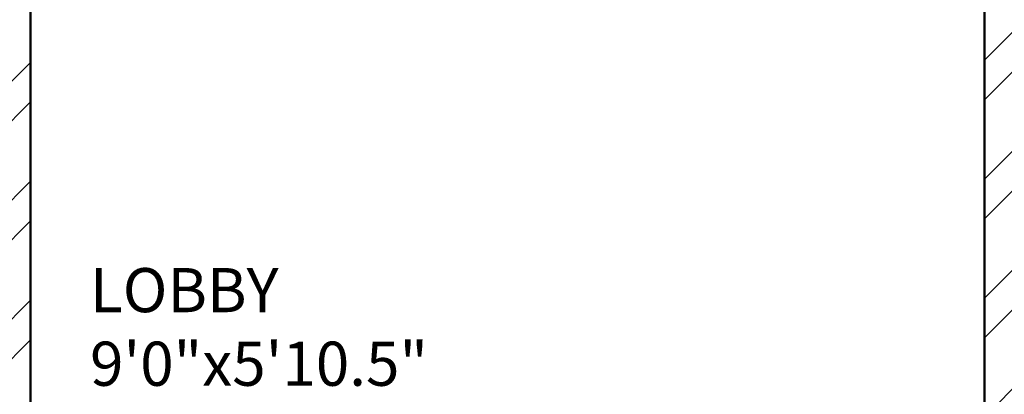
# Model space of a CAD drawing. Units: inches. Extents: x 963 to 2075, y 289 to 2657.
# Tile 68 of 98: x 1399 to 1511, y 2117 to 2160. Entities that reach past the tile are written whole.
import ezdxf

# ---------------------------------------------------------------- set-up
doc = ezdxf.new("R2010")
doc.units = ezdxf.units.IN
for name, color, linetype, lineweight in [('A-AREA-IDEN', 7, 'Continuous', 18), ('A-WALL', 7, 'Continuous', 50), ('A-WALL-PATT', 8, 'Continuous', 13)]:
    doc.layers.add(name, color=color, linetype=linetype, lineweight=lineweight)
doc.styles.get("Standard").update_dxf_attribs({"font": 'arial.ttf'})

msp = doc.modelspace()

# ---------------------------------------------------------------- hatches: boundary and pattern name
at = {"layer": 'A-WALL-PATT'}
h = msp.add_hatch(dxfattribs=at)
h.set_pattern_fill('ANSI32', color=256)
h.paths.add_polyline_path([(1296.92, 2558.32), (1203.92, 2558.32), (1203.92, 2493.82), (1191.53, 2493.82), (1191.53, 2489.32), (1211.06, 2489.32), (1211.06, 2492.02), (1211.06, 2493.82), (1208.42, 2493.82), (1208.42, 2553.82), (1292.42, 2553.82), (1292.42, 2538.86), (1296.92, 2538.86)])
h.paths.add_polyline_path([(1442.42, 2558.32), (1349.42, 2558.32), (1349.42, 2538.94), (1353.92, 2538.94), (1353.92, 2553.82), (1437.92, 2553.82), (1437.92, 2493.82), (1434.54, 2493.82), (1434.54, 2489.32), (1448.31, 2489.32), (1448.31, 2491.57), (1448.31, 2493.82), (1442.42, 2493.82)])
h.paths.add_polyline_path([(1415.55, 2491.57), (1415.55, 2493.82), (1340.94, 2493.82), (1340.94, 2489.32), (1371.92, 2489.32), (1371.92, 2378.32), (1367.6, 2378.32), (1367.6, 2373.82), (1371.92, 2373.82), (1371.92, 2355.19), (1376.42, 2355.19), (1376.42, 2489.32), (1415.55, 2489.32)])
h.paths.add_polyline_path([(1304.94, 2491.57), (1304.94, 2493.82), (1296.92, 2493.82), (1296.92, 2514.86), (1292.42, 2514.86), (1292.42, 2493.82), (1232.81, 2493.82), (1232.81, 2489.32), (1256.42, 2489.32), (1256.42, 2327.32), (1253.71, 2327.32), (1253.71, 2322.82), (1328.42, 2322.82), (1328.42, 2331.15), (1323.92, 2331.15), (1323.92, 2327.32), (1260.92, 2327.32), (1260.92, 2373.82), (1323.92, 2373.82), (1323.92, 2357.81), (1328.42, 2357.81), (1328.42, 2373.82), (1346.01, 2373.82), (1346.01, 2376.07), (1346.01, 2378.32), (1260.92, 2378.32), (1260.92, 2489.32), (1304.94, 2489.32)])
h.paths.add_polyline_path([(1226.65, 2327.32), (1124.42, 2327.32), (1124.42, 2347.45), (1119.92, 2347.45), (1119.92, 2322.82), (1163.42, 2322.82), (1163.42, 2305.43), (1165.67, 2305.43), (1167.92, 2305.43), (1167.92, 2322.82), (1226.65, 2322.82), (1226.65, 2325.07)])
h.paths.add_polyline_path([(1095.92, 2489.32), (1124.42, 2489.32), (1131.53, 2489.32), (1131.53, 2491.57), (1131.53, 2493.82), (1119.92, 2493.82), (1091.42, 2493.82), (1091.42, 2417.32), (1095.92, 2417.32), (1119.92, 2417.32), (1119.92, 2407.45), (1124.42, 2407.45), (1124.42, 2421.82), (1095.92, 2421.82)])
h.paths.add_polyline_path([(1512.92, 2558.32), (1508.42, 2558.32), (1508.42, 2493.82), (1503.4, 2493.82), (1503.4, 2489.32), (1508.42, 2489.32), (1508.42, 2327.32), (1376.42, 2327.32), (1376.42, 2330.27), (1371.92, 2330.27), (1371.92, 2298.74), (1376.42, 2298.74), (1376.42, 2322.82), (1508.42, 2322.82), (1508.42, 2165.32), (1504.26, 2165.32), (1504.26, 2160.82), (1508.42, 2160.82), (1508.42, 2108.32), (1512.92, 2108.32), (1512.92, 2160.82), (1516.18, 2160.82), (1516.18, 2163.07), (1516.18, 2165.32), (1512.92, 2165.32), (1512.92, 2322.82), (1644.92, 2322.82), (1644.92, 2298.74), (1649.42, 2298.74), (1649.42, 2322.82), (1649.42, 2330.94), (1647.17, 2330.94), (1644.92, 2330.94), (1644.92, 2327.32), (1512.92, 2327.32), (1512.92, 2489.32), (1516.76, 2489.32), (1516.76, 2491.57), (1516.76, 2493.82), (1512.92, 2493.82)])
h.paths.add_polyline_path([(1671.92, 2558.32), (1578.92, 2558.32), (1578.92, 2493.82), (1573.53, 2493.82), (1573.53, 2489.32), (1586.54, 2489.32), (1586.54, 2491.57), (1586.54, 2493.82), (1583.42, 2493.82), (1583.42, 2553.82), (1667.42, 2553.82), (1667.42, 2541.11), (1671.92, 2541.11)])
h.paths.add_polyline_path([(1681.26, 2493.82), (1671.92, 2493.82), (1671.92, 2517.11), (1667.42, 2517.11), (1667.42, 2493.82), (1610.22, 2493.82), (1610.22, 2489.32), (1644.92, 2489.32), (1644.92, 2357.87), (1649.42, 2357.87), (1649.42, 2373.82), (1652.2, 2373.82), (1652.2, 2375.83), (1652.2, 2378.32), (1649.42, 2378.32), (1649.42, 2489.32), (1681.26, 2489.32), (1681.26, 2491.57)])
h.paths.add_polyline_path([(1821.92, 2558.32), (1728.92, 2558.32), (1728.92, 2541), (1733.42, 2541), (1733.42, 2553.82), (1817.42, 2553.82), (1817.42, 2493.82), (1813.51, 2493.82), (1813.51, 2489.32), (1830.08, 2489.32), (1830.08, 2491.57), (1830.08, 2493.82), (1821.92, 2493.82)])
h.paths.add_polyline_path([(1794.24, 2493.82), (1717.26, 2493.82), (1717.26, 2489.32), (1760.42, 2489.32), (1760.42, 2378.32), (1674.4, 2378.32), (1674.4, 2373.82), (1692.92, 2373.82), (1692.92, 2356.95), (1697.42, 2356.95), (1697.42, 2373.82), (1760.42, 2373.82), (1760.42, 2327.32), (1697.42, 2327.32), (1697.42, 2333.34), (1692.92, 2333.34), (1692.92, 2322.82), (1768.04, 2322.82), (1768.04, 2325.07), (1768.04, 2327.32), (1764.92, 2327.32), (1764.92, 2489.32), (1794.24, 2489.32)])
h.paths.add_polyline_path([(1733.42, 2517), (1728.92, 2517), (1728.92, 2493.82), (1733.42, 2493.82)], flags=17)
h.paths.add_polyline_path([(1929.92, 2493.82), (1890.08, 2493.82), (1890.08, 2489.32), (1896.92, 2489.32), (1925.42, 2489.32), (1925.42, 2421.82), (1896.92, 2421.82), (1896.92, 2408.32), (1901.42, 2408.32), (1901.42, 2417.32), (1925.42, 2417.32), (1929.92, 2417.32)])
h.paths.add_polyline_path([(1901.42, 2348.32), (1896.92, 2348.32), (1896.92, 2327.32), (1800.42, 2327.32), (1800.42, 2322.82), (1853.42, 2322.82), (1853.42, 2309.45), (1857.92, 2309.45), (1857.92, 2322.82), (1901.42, 2322.82)])
h.paths.add_polyline_path([(1857.92, 2249.45), (1853.42, 2249.45), (1853.42, 2214.82), (1686.31, 2214.82), (1686.31, 2210.32), (1853.42, 2210.32), (1853.42, 2202.13), (1857.92, 2202.13), (1857.92, 2210.32)])
h.paths.add_polyline_path([(1857.92, 2142.13), (1853.42, 2142.13), (1853.42, 2115.42), (1841.42, 2115.42), (1841.42, 2088.53), (1841.42, 2046.95), (1845.92, 2046.95), (1845.92, 2110.92), (1905.92, 2110.92), (1905.92, 2092.52), (1910.42, 2092.52), (1910.42, 2115.42), (1857.92, 2115.42)])
h.paths.add_polyline_path([(1532.44, 1482.34), (1573.46, 1482.34), (1573.46, 1501), (1532.44, 1501)], flags=9)
h.paths.add_polyline_path([(1438.66, 1486.3), (1479.68, 1486.3), (1479.68, 1504.96), (1438.66, 1504.96)], flags=9)
h.paths.add_polyline_path([(1411.22, 1365.31), (1659.14, 1365.31), (1659.14, 1402.4), (1411.22, 1402.4)], flags=9)
h.paths.add_polyline_path([(1185.67, 2296.3), (1248.16, 2296.3), (1248.16, 2314.95), (1185.67, 2314.95)], flags=9)
h.paths.add_polyline_path([(1177.31, 2187.35), (1216.15, 2187.35), (1216.15, 2206.01), (1177.31, 2206.01)], flags=9)
h.paths.add_polyline_path([(1295.1, 1602.08), (1328.26, 1602.08), (1328.26, 1620.74), (1295.1, 1620.74)], flags=9)
h.paths.add_polyline_path([(1525.13, 2005.99), (1558.39, 2005.99), (1558.39, 2024.65), (1525.13, 2024.65)], flags=9)
h.paths.add_polyline_path([(1459.61, 1977.13), (1472.19, 1977.13), (1472.19, 1987.43), (1459.61, 1987.43)], flags=9)
h.paths.add_polyline_path([(1467.81, 2053.68), (1480.02, 2053.68), (1480.02, 2063.98), (1467.81, 2063.98)], flags=9)
h.paths.add_polyline_path([(1555.18, 2119.02), (1584.56, 2119.02), (1584.56, 2137.68), (1555.18, 2137.68)], flags=25)
h.paths.add_polyline_path([(1405.39, 2115.29), (1444.48, 2115.29), (1444.48, 2133.95), (1405.39, 2133.95)], flags=25)
h.paths.add_polyline_path([(1698.48, 2004.26), (1727.69, 2004.26), (1727.69, 2022.92), (1698.48, 2022.92)], flags=9)
h.paths.add_polyline_path([(1612.16, 1972.86), (1629.02, 1972.86), (1629.02, 1983.16), (1612.16, 1983.16)], flags=9)
h.paths.add_polyline_path([(1608.29, 2060.04), (1625.15, 2060.04), (1625.15, 2070.34), (1608.29, 2070.34)], flags=9)
h.paths.add_polyline_path([(1527.95, 1684.4), (1566.79, 1684.4), (1566.79, 1703.06), (1527.95, 1703.06)], flags=9)
h.paths.add_polyline_path([(1422.79, 1683.59), (1461.63, 1683.59), (1461.63, 1702.25), (1422.79, 1702.25)], flags=9)
h.paths.add_polyline_path([(1531.26, 1732.46), (1574.01, 1732.46), (1574.01, 1751.12), (1531.26, 1751.12)], flags=9)
h.paths.add_polyline_path([(1402.87, 1732.85), (1439.8, 1732.85), (1439.8, 1751.5), (1402.87, 1751.5)], flags=9)
h.paths.add_polyline_path([(1243.12, 1923.13), (1281.96, 1923.13), (1281.96, 1941.79), (1243.12, 1941.79)], flags=9)
h.paths.add_polyline_path([(1181.75, 1792.27), (1244.24, 1792.27), (1244.24, 1810.93), (1181.75, 1810.93)], flags=9)
h.paths.add_polyline_path([(1265.82, 1670.3), (1316.07, 1670.3), (1316.07, 1688.96), (1265.82, 1688.96)], flags=9)
h.paths.add_polyline_path([(1140.26, 1676.05), (1179.1, 1676.05), (1179.1, 1694.71), (1140.26, 1694.71)], flags=9)
h.paths.add_polyline_path([(1107.49, 1490.89), (1143.37, 1490.89), (1143.37, 1509.55), (1107.49, 1509.55)], flags=9)
h.paths.add_polyline_path([(1217.58, 1483.9), (1246.74, 1483.9), (1246.74, 1502.56), (1217.58, 1502.56)], flags=9)
h.paths.add_polyline_path([(1389.21, 1486.92), (1418.37, 1486.92), (1418.37, 1505.58), (1389.21, 1505.58)], flags=9)
h.paths.add_polyline_path([(1672.21, 1602.08), (1705.37, 1602.08), (1705.37, 1620.74), (1672.21, 1620.74)], flags=9)
h.paths.add_polyline_path([(1752.08, 1522.64), (1781.24, 1522.64), (1781.24, 1541.3), (1752.08, 1541.3)], flags=9)
h.paths.add_polyline_path([(1848.27, 1491.26), (1884.16, 1491.26), (1884.16, 1509.92), (1848.27, 1509.92)], flags=9)
h.paths.add_polyline_path([(1822.47, 1685.62), (1861.31, 1685.62), (1861.31, 1704.28), (1822.47, 1704.28)], flags=9)
h.paths.add_polyline_path([(1713.19, 1672.23), (1763.44, 1672.23), (1763.44, 1690.89), (1713.19, 1690.89)], flags=9)
h.paths.add_polyline_path([(1736.62, 1790.58), (1799.11, 1790.58), (1799.11, 1809.24), (1736.62, 1809.24)], flags=9)
h.paths.add_polyline_path([(1691.49, 1916.36), (1730.33, 1916.36), (1730.33, 1935.01), (1691.49, 1935.01)], flags=9)
h.paths.add_polyline_path([(1764.87, 1973.92), (1794.31, 1973.92), (1794.31, 1992.58), (1764.87, 1992.58)], flags=9)
h.paths.add_polyline_path([(1767.85, 2034.02), (1797.29, 2034.02), (1797.29, 2052.67), (1767.85, 2052.67)], flags=9)
h.paths.add_polyline_path([(1851.59, 2060.33), (1880.75, 2060.33), (1880.75, 2078.99), (1851.59, 2078.99)], flags=25)
h.paths.add_polyline_path([(1688.49, 2086.87), (1727.33, 2086.87), (1727.33, 2105.53), (1688.49, 2105.53)], flags=9)
h.paths.add_polyline_path([(1537.74, 2293.58), (1580.49, 2293.58), (1580.49, 2312.24), (1537.74, 2312.24)], flags=25)
h.paths.add_polyline_path([(1425.59, 2296.11), (1468.34, 2296.11), (1468.34, 2314.77), (1425.59, 2314.77)], flags=25)
h.paths.add_polyline_path([(1278.52, 2004.18), (1307.72, 2004.18), (1307.72, 2022.84), (1278.52, 2022.84)], flags=9)
h.paths.add_polyline_path([(1193.28, 1973.63), (1222.72, 1973.63), (1222.72, 1992.29), (1193.28, 1992.29)], flags=9)
h.paths.add_polyline_path([(1192.41, 2040.58), (1221.84, 2040.58), (1221.84, 2059.23), (1192.41, 2059.23)], flags=9)
h.paths.add_polyline_path([(1130.6, 1951.39), (1159.76, 1951.39), (1159.76, 1970.05), (1130.6, 1970.05)], flags=9)
h.paths.add_polyline_path([(1132.83, 2052.49), (1161.98, 2052.49), (1161.98, 2071.15), (1132.83, 2071.15)], flags=9)
h.paths.add_polyline_path([(1265.13, 2334.62), (1315.38, 2334.62), (1315.38, 2353.28), (1265.13, 2353.28)], flags=25)
h.paths.add_polyline_path([(1136.74, 2330.79), (1175.58, 2330.79), (1175.58, 2349.44), (1136.74, 2349.44)], flags=9)
h.paths.add_polyline_path([(1287.42, 2417.2), (1320.58, 2417.2), (1320.58, 2435.86), (1287.42, 2435.86)], flags=25)
h.paths.add_polyline_path([(1430.99, 2329.16), (1469.83, 2329.16), (1469.83, 2347.82), (1430.99, 2347.82)], flags=25)
h.paths.add_polyline_path([(1525.42, 2329.21), (1564.26, 2329.21), (1564.26, 2347.87), (1525.42, 2347.87)], flags=25)
h.paths.add_polyline_path([(1684.52, 2382.8), (1717.68, 2382.8), (1717.68, 2401.46), (1684.52, 2401.46)], flags=25)
h.paths.add_polyline_path([(1704.81, 2340.29), (1755.05, 2340.29), (1755.05, 2358.95), (1704.81, 2358.95)], flags=25)
h.paths.add_polyline_path([(1694.11, 2287.76), (1756.6, 2287.76), (1756.6, 2306.41), (1694.11, 2306.41)], flags=9)
h.paths.add_polyline_path([(1815.78, 2329.86), (1854.62, 2329.86), (1854.62, 2348.52), (1815.78, 2348.52)], flags=9)
h.paths.add_polyline_path([(1842.87, 2514.26), (1878.76, 2514.26), (1878.76, 2532.91), (1842.87, 2532.91)], flags=9)
h.paths.add_polyline_path([(1769.51, 2531.45), (1798.67, 2531.45), (1798.67, 2550.1), (1769.51, 2550.1)], flags=25)
h.paths.add_polyline_path([(1594.77, 2518.47), (1623.93, 2518.47), (1623.93, 2537.13), (1594.77, 2537.13)], flags=25)
h.paths.add_polyline_path([(1520.72, 2516.18), (1556.61, 2516.18), (1556.61, 2534.84), (1520.72, 2534.84)], flags=25)
h.paths.add_polyline_path([(1464.46, 2516.69), (1500.34, 2516.69), (1500.34, 2535.35), (1464.46, 2535.35)], flags=25)
h.paths.add_polyline_path([(1365.7, 2528.97), (1394.85, 2528.97), (1394.85, 2547.63), (1365.7, 2547.63)], flags=25)
h.paths.add_polyline_path([(1222.84, 2516.23), (1252, 2516.23), (1252, 2534.89), (1222.84, 2534.89)], flags=25)
h.paths.add_polyline_path([(1104.55, 2509.6), (1140.43, 2509.6), (1140.43, 2528.26), (1104.55, 2528.26)], flags=9)
h = msp.add_hatch(dxfattribs=at)
h.set_pattern_fill('ANSI32', color=256)
h.paths.add_polyline_path([(1335.97, 2212.57), (1335.97, 2214.82), (1167.92, 2214.82), (1167.92, 2245.43), (1163.42, 2245.43), (1163.42, 2210.32), (1163.42, 2194.81), (1167.92, 2194.81), (1167.92, 2210.32), (1335.97, 2210.32)])
h.paths.add_polyline_path([(1532.44, 1482.34), (1573.46, 1482.34), (1573.46, 1501), (1532.44, 1501)], flags=9)
h.paths.add_polyline_path([(1438.66, 1486.3), (1479.68, 1486.3), (1479.68, 1504.96), (1438.66, 1504.96)], flags=9)
h.paths.add_polyline_path([(1411.22, 1365.31), (1659.14, 1365.31), (1659.14, 1402.4), (1411.22, 1402.4)], flags=9)
h.paths.add_polyline_path([(1185.67, 2296.3), (1248.16, 2296.3), (1248.16, 2314.95), (1185.67, 2314.95)], flags=9)
h.paths.add_polyline_path([(1177.31, 2187.35), (1216.15, 2187.35), (1216.15, 2206.01), (1177.31, 2206.01)], flags=9)
h.paths.add_polyline_path([(1295.1, 1602.08), (1328.26, 1602.08), (1328.26, 1620.74), (1295.1, 1620.74)], flags=9)
h.paths.add_polyline_path([(1525.13, 2005.99), (1558.39, 2005.99), (1558.39, 2024.65), (1525.13, 2024.65)], flags=9)
h.paths.add_polyline_path([(1459.61, 1977.13), (1472.19, 1977.13), (1472.19, 1987.43), (1459.61, 1987.43)], flags=9)
h.paths.add_polyline_path([(1467.81, 2053.68), (1480.02, 2053.68), (1480.02, 2063.98), (1467.81, 2063.98)], flags=9)
h.paths.add_polyline_path([(1555.18, 2119.02), (1584.56, 2119.02), (1584.56, 2137.68), (1555.18, 2137.68)], flags=9)
h.paths.add_polyline_path([(1405.39, 2115.29), (1444.48, 2115.29), (1444.48, 2133.95), (1405.39, 2133.95)], flags=9)
h.paths.add_polyline_path([(1698.48, 2004.26), (1727.69, 2004.26), (1727.69, 2022.92), (1698.48, 2022.92)], flags=9)
h.paths.add_polyline_path([(1612.16, 1972.86), (1629.02, 1972.86), (1629.02, 1983.16), (1612.16, 1983.16)], flags=9)
h.paths.add_polyline_path([(1608.29, 2060.04), (1625.15, 2060.04), (1625.15, 2070.34), (1608.29, 2070.34)], flags=9)
h.paths.add_polyline_path([(1527.95, 1684.4), (1566.79, 1684.4), (1566.79, 1703.06), (1527.95, 1703.06)], flags=9)
h.paths.add_polyline_path([(1422.79, 1683.59), (1461.63, 1683.59), (1461.63, 1702.25), (1422.79, 1702.25)], flags=9)
h.paths.add_polyline_path([(1531.26, 1732.46), (1574.01, 1732.46), (1574.01, 1751.12), (1531.26, 1751.12)], flags=9)
h.paths.add_polyline_path([(1402.87, 1732.85), (1439.8, 1732.85), (1439.8, 1751.5), (1402.87, 1751.5)], flags=9)
h.paths.add_polyline_path([(1243.12, 1923.13), (1281.96, 1923.13), (1281.96, 1941.79), (1243.12, 1941.79)], flags=9)
h.paths.add_polyline_path([(1181.75, 1792.27), (1244.24, 1792.27), (1244.24, 1810.93), (1181.75, 1810.93)], flags=9)
h.paths.add_polyline_path([(1265.82, 1670.3), (1316.07, 1670.3), (1316.07, 1688.96), (1265.82, 1688.96)], flags=9)
h.paths.add_polyline_path([(1140.26, 1676.05), (1179.1, 1676.05), (1179.1, 1694.71), (1140.26, 1694.71)], flags=9)
h.paths.add_polyline_path([(1107.49, 1490.89), (1143.37, 1490.89), (1143.37, 1509.55), (1107.49, 1509.55)], flags=9)
h.paths.add_polyline_path([(1217.58, 1483.9), (1246.74, 1483.9), (1246.74, 1502.56), (1217.58, 1502.56)], flags=9)
h.paths.add_polyline_path([(1389.21, 1486.92), (1418.37, 1486.92), (1418.37, 1505.58), (1389.21, 1505.58)], flags=9)
h.paths.add_polyline_path([(1672.21, 1602.08), (1705.37, 1602.08), (1705.37, 1620.74), (1672.21, 1620.74)], flags=9)
h.paths.add_polyline_path([(1752.08, 1522.64), (1781.24, 1522.64), (1781.24, 1541.3), (1752.08, 1541.3)], flags=9)
h.paths.add_polyline_path([(1848.27, 1491.26), (1884.16, 1491.26), (1884.16, 1509.92), (1848.27, 1509.92)], flags=9)
h.paths.add_polyline_path([(1822.47, 1685.62), (1861.31, 1685.62), (1861.31, 1704.28), (1822.47, 1704.28)], flags=9)
h.paths.add_polyline_path([(1713.19, 1672.23), (1763.44, 1672.23), (1763.44, 1690.89), (1713.19, 1690.89)], flags=9)
h.paths.add_polyline_path([(1736.62, 1790.58), (1799.11, 1790.58), (1799.11, 1809.24), (1736.62, 1809.24)], flags=9)
h.paths.add_polyline_path([(1691.49, 1916.36), (1730.33, 1916.36), (1730.33, 1935.01), (1691.49, 1935.01)], flags=9)
h.paths.add_polyline_path([(1764.87, 1973.92), (1794.31, 1973.92), (1794.31, 1992.58), (1764.87, 1992.58)], flags=9)
h.paths.add_polyline_path([(1767.85, 2034.02), (1797.29, 2034.02), (1797.29, 2052.67), (1767.85, 2052.67)], flags=9)
h.paths.add_polyline_path([(1851.59, 2060.33), (1880.75, 2060.33), (1880.75, 2078.99), (1851.59, 2078.99)], flags=9)
h.paths.add_polyline_path([(1688.49, 2086.87), (1727.33, 2086.87), (1727.33, 2105.53), (1688.49, 2105.53)], flags=9)
h.paths.add_polyline_path([(1537.74, 2293.58), (1580.49, 2293.58), (1580.49, 2312.24), (1537.74, 2312.24)], flags=9)
h.paths.add_polyline_path([(1425.59, 2296.11), (1468.34, 2296.11), (1468.34, 2314.77), (1425.59, 2314.77)], flags=9)
h.paths.add_polyline_path([(1278.52, 2004.18), (1307.72, 2004.18), (1307.72, 2022.84), (1278.52, 2022.84)], flags=9)
h.paths.add_polyline_path([(1193.28, 1973.63), (1222.72, 1973.63), (1222.72, 1992.29), (1193.28, 1992.29)], flags=9)
h.paths.add_polyline_path([(1192.41, 2040.58), (1221.84, 2040.58), (1221.84, 2059.23), (1192.41, 2059.23)], flags=9)
h.paths.add_polyline_path([(1130.6, 1951.39), (1159.76, 1951.39), (1159.76, 1970.05), (1130.6, 1970.05)], flags=9)
h.paths.add_polyline_path([(1132.83, 2052.49), (1161.98, 2052.49), (1161.98, 2071.15), (1132.83, 2071.15)], flags=9)
h.paths.add_polyline_path([(1265.13, 2334.62), (1315.38, 2334.62), (1315.38, 2353.28), (1265.13, 2353.28)], flags=9)
h.paths.add_polyline_path([(1136.74, 2330.79), (1175.58, 2330.79), (1175.58, 2349.44), (1136.74, 2349.44)], flags=9)
h.paths.add_polyline_path([(1287.42, 2417.2), (1320.58, 2417.2), (1320.58, 2435.86), (1287.42, 2435.86)], flags=9)
h.paths.add_polyline_path([(1430.99, 2329.16), (1469.83, 2329.16), (1469.83, 2347.82), (1430.99, 2347.82)], flags=9)
h.paths.add_polyline_path([(1525.42, 2329.21), (1564.26, 2329.21), (1564.26, 2347.87), (1525.42, 2347.87)], flags=9)
h.paths.add_polyline_path([(1684.52, 2382.8), (1717.68, 2382.8), (1717.68, 2401.46), (1684.52, 2401.46)], flags=9)
h.paths.add_polyline_path([(1704.81, 2340.29), (1755.05, 2340.29), (1755.05, 2358.95), (1704.81, 2358.95)], flags=9)
h.paths.add_polyline_path([(1694.11, 2287.76), (1756.6, 2287.76), (1756.6, 2306.41), (1694.11, 2306.41)], flags=9)
h.paths.add_polyline_path([(1815.78, 2329.86), (1854.62, 2329.86), (1854.62, 2348.52), (1815.78, 2348.52)], flags=9)
h.paths.add_polyline_path([(1842.87, 2514.26), (1878.76, 2514.26), (1878.76, 2532.91), (1842.87, 2532.91)], flags=9)
h.paths.add_polyline_path([(1769.51, 2531.45), (1798.67, 2531.45), (1798.67, 2550.1), (1769.51, 2550.1)], flags=9)
h.paths.add_polyline_path([(1594.77, 2518.47), (1623.93, 2518.47), (1623.93, 2537.13), (1594.77, 2537.13)], flags=9)
h.paths.add_polyline_path([(1520.72, 2516.18), (1556.61, 2516.18), (1556.61, 2534.84), (1520.72, 2534.84)], flags=9)
h.paths.add_polyline_path([(1464.46, 2516.69), (1500.34, 2516.69), (1500.34, 2535.35), (1464.46, 2535.35)], flags=9)
h.paths.add_polyline_path([(1365.7, 2528.97), (1394.85, 2528.97), (1394.85, 2547.63), (1365.7, 2547.63)], flags=9)
h.paths.add_polyline_path([(1222.84, 2516.23), (1252, 2516.23), (1252, 2534.89), (1222.84, 2534.89)], flags=9)
h.paths.add_polyline_path([(1104.55, 2509.6), (1140.43, 2509.6), (1140.43, 2528.26), (1104.55, 2528.26)], flags=9)
h = msp.add_hatch(dxfattribs=at)
h.set_pattern_fill('ANSI32', color=256)
h.paths.add_polyline_path([(1473.61, 2163.07), (1473.61, 2165.32), (1376.42, 2165.32), (1376.42, 2227.98), (1371.92, 2227.98), (1371.92, 2214.82), (1368.41, 2214.82), (1368.41, 2210.32), (1371.92, 2210.32), (1371.92, 2160.82), (1395.92, 2160.82), (1395.92, 2090.32), (1217.34, 2090.32), (1217.34, 2085.82), (1395.92, 2085.82), (1458.92, 2085.82), (1458.92, 2108.32), (1454.42, 2108.32), (1454.42, 2090.32), (1400.42, 2090.32), (1400.42, 2160.82), (1473.61, 2160.82)])
h.paths.add_polyline_path([(1649.42, 2210.32), (1653.23, 2210.32), (1653.23, 2214.82), (1649.42, 2214.82), (1649.42, 2227.98), (1644.92, 2227.98), (1644.92, 2165.32), (1550.1, 2165.32), (1550.1, 2160.82), (1620.92, 2160.82), (1620.92, 2112.82), (1555.45, 2112.82), (1555.45, 2108.32), (1584.33, 2108.32), (1584.33, 2084.92), (1588.83, 2084.92), (1588.83, 2108.32), (1625.42, 2108.32), (1667.95, 2108.32), (1667.95, 2022.67), (1588.83, 2022.67), (1588.83, 2047.41), (1584.33, 2047.41), (1584.33, 1996), (1588.83, 1996), (1588.83, 2018.32), (1667.95, 2018.17), (1667.95, 1928.32), (1625.42, 1928.32), (1625.42, 1923.82), (1672.45, 1923.82), (1672.45, 1928.32), (1672.45, 1946.66), (1785.45, 1946.66), (1785.45, 1951.16), (1743.03, 1951.16), (1743.03, 2017.92), (1841.42, 2017.92), (1841.42, 2014.77), (1845.92, 2014.77), (1845.92, 2017.92), (1905.92, 2017.92), (1905.92, 1987.51), (1910.42, 1987.51), (1910.42, 2022.42), (1910.42, 2068.52), (1905.92, 2068.52), (1905.92, 2022.42), (1845.92, 2022.42), (1845.92, 2025.85), (1843.67, 2025.85), (1841.42, 2025.85), (1841.42, 2022.42), (1743.03, 2022.42), (1743.03, 2084.03), (1768.45, 2084.03), (1785.45, 2084.03), (1785.45, 2088.53), (1672.45, 2088.53), (1672.45, 2112.82), (1667.95, 2112.82), (1625.42, 2112.82), (1625.42, 2160.82), (1649.42, 2160.82)])
h.paths.add_polyline_path([(1672.45, 2084.03), (1738.53, 2084.03), (1738.53, 1951.16), (1672.45, 1951.16)], flags=16)
h.paths.add_polyline_path([(1672.45, 2084.03), (1738.53, 2084.03), (1705.49, 2017.6)], flags=0)
h.paths.add_polyline_path([(1262.77, 2085.82), (1258.27, 2085.82), (1258.27, 2023.28), (1184.42, 2023.28), (1184.42, 2018.78), (1258.27, 2018.78), (1258.27, 1950.82), (1262.77, 1950.82)])
h.paths.add_polyline_path([(1312.27, 2085.82), (1307.77, 2085.82), (1307.77, 1950.82), (1312.27, 1950.82)])
h.paths.add_polyline_path([(1458.92, 1950.82), (1395.92, 1950.82), (1216.57, 1950.82), (1216.57, 1946.32), (1346.42, 1946.32), (1395.92, 1946.32), (1395.92, 1875.82), (1371.92, 1875.82), (1371.92, 1826.32), (1368.93, 1826.32), (1368.93, 1821.82), (1371.92, 1821.82), (1371.92, 1813.62), (1376.42, 1813.62), (1376.42, 1871.32), (1474.5, 1871.32), (1474.5, 1873.57), (1474.5, 1875.82), (1400.42, 1875.82), (1400.42, 1946.32), (1454.42, 1946.32), (1454.42, 1928.32), (1458.92, 1928.32)])
h.paths.add_polyline_path([(1184.42, 2120.78), (1167.92, 2120.78), (1167.92, 2134.81), (1165.67, 2134.81), (1163.42, 2134.81), (1163.42, 2120.78), (1119.92, 2120.78), (1119.92, 2098.1), (1124.42, 2098.1), (1124.42, 2116.28), (1167.92, 2116.28), (1179.92, 2116.28), (1179.92, 2045.92), (1184.42, 2045.92), (1184.42, 2090.32), (1184.42, 2116.28)])
h.paths.add_polyline_path([(1124.42, 2018.78), (1179.92, 2018.78), (1179.92, 2016.29), (1184.42, 2016.29), (1184.42, 2023.28), (1184.42, 2026.59), (1182.17, 2026.59), (1179.92, 2026.59), (1179.92, 2023.28), (1124.42, 2023.28), (1124.42, 2074.1), (1119.92, 2074.1), (1119.92, 2018.78), (1119.92, 1979.63), (1124.42, 1979.63)])
h.paths.add_polyline_path([(1184.42, 1925.78), (1184.42, 1946.32), (1184.42, 1996.07), (1182.17, 1996.07), (1179.92, 1996.07), (1179.92, 1925.78), (1124.42, 1925.78), (1124.42, 1955.63), (1119.92, 1955.5), (1119.92, 1921.28), (1158.92, 1921.28), (1158.92, 1909.98), (1163.42, 1909.98), (1163.42, 1921.28), (1184.42, 1921.28)])
h.paths.add_polyline_path([(1341.45, 1826.32), (1163.42, 1826.32), (1163.42, 1849.98), (1158.92, 1849.98), (1158.92, 1821.82), (1158.92, 1804.03), (1163.42, 1804.03), (1163.42, 1821.82), (1341.45, 1821.82)])
h.paths.add_polyline_path([(1222.98, 1713.82), (1163.42, 1713.82), (1163.42, 1744.03), (1161.17, 1744.03), (1158.92, 1744.03), (1158.92, 1713.82), (1119.92, 1713.82), (1119.92, 1694.65), (1124.42, 1694.65), (1124.42, 1709.32), (1158.92, 1709.32), (1222.98, 1709.32)])
h.paths.add_polyline_path([(1328.42, 1713.82), (1252.04, 1713.82), (1252.04, 1711.57), (1252.04, 1709.32), (1256.42, 1709.32), (1256.42, 1547.32), (1232.94, 1547.32), (1232.94, 1545.07), (1232.94, 1542.82), (1292.42, 1542.82), (1292.42, 1527.63), (1296.92, 1527.63), (1296.92, 1542.82), (1299.46, 1542.82), (1299.46, 1547.32), (1260.92, 1547.32), (1260.92, 1658.32), (1343.66, 1658.32), (1343.66, 1660.57), (1343.66, 1662.82), (1328.42, 1662.82), (1328.42, 1676.59), (1327.4, 1676.59), (1323.92, 1676.59), (1323.92, 1662.82), (1260.92, 1662.82), (1260.92, 1709.32), (1323.92, 1709.32), (1323.92, 1699.85), (1328.42, 1699.85)])
h.paths.add_polyline_path([(1649.42, 1875.82), (1625.42, 1875.82), (1625.42, 1928.32), (1620.92, 1928.32), (1588.83, 1928.32), (1588.83, 1950.59), (1584.33, 1950.59), (1584.33, 1928.32), (1555.45, 1928.32), (1555.45, 1923.82), (1620.92, 1923.82), (1620.92, 1875.82), (1548.95, 1875.82), (1548.95, 1873.57), (1548.95, 1871.32), (1644.92, 1871.32), (1644.92, 1813.62), (1649.42, 1813.62), (1649.42, 1821.82), (1652.04, 1821.82), (1652.04, 1824.07), (1652.04, 1826.32), (1649.42, 1826.32)])
h.paths.add_polyline_path([(1512.92, 1871.32), (1516.48, 1871.32), (1516.48, 1875.82), (1512.92, 1875.82), (1512.92, 1923.82), (1512.92, 1928.32), (1512.92, 1930.83), (1508.42, 1930.83), (1508.42, 1875.82), (1504.41, 1875.82), (1504.41, 1871.32), (1508.42, 1871.32), (1508.42, 1713.82), (1376.42, 1713.82), (1376.42, 1743.32), (1371.92, 1743.32), (1371.92, 1709.32), (1371.92, 1706.01), (1376.42, 1706.01), (1376.42, 1709.32), (1508.42, 1709.32), (1508.42, 1547.32), (1501.87, 1547.32), (1501.87, 1542.82), (1508.42, 1542.82), (1508.42, 1482.82), (1508.42, 1436.32), (1512.92, 1436.32), (1512.92, 1542.82), (1519.32, 1542.82), (1519.32, 1545.07), (1519.32, 1547.32), (1512.92, 1547.32), (1512.92, 1709.32), (1644.92, 1709.32), (1644.92, 1707.55), (1649.42, 1707.55), (1649.42, 1709.32), (1649.42, 1743.32), (1644.92, 1743.32), (1644.92, 1713.82), (1512.92, 1713.82)])
h.paths.add_polyline_path([(1129.88, 1545.07), (1129.88, 1547.32), (1124.42, 1547.32), (1095.92, 1547.32), (1095.92, 1614.82), (1124.42, 1614.82), (1124.42, 1619.32), (1095.92, 1619.32), (1091.42, 1619.32), (1091.42, 1542.82), (1095.92, 1542.82), (1119.92, 1542.82), (1129.88, 1542.82)])
h.paths.add_polyline_path([(1208.42, 1542.82), (1211.74, 1542.82), (1211.74, 1547.32), (1198.85, 1547.32), (1198.85, 1542.82), (1203.92, 1542.82), (1203.92, 1478.32), (1208.42, 1478.32), (1296.92, 1478.32), (1296.92, 1503.63), (1292.42, 1503.63), (1292.42, 1482.82), (1208.42, 1482.82)])
h.paths.add_polyline_path([(1430.42, 1542.82), (1435.7, 1542.82), (1435.7, 1545.07), (1435.7, 1547.32), (1422.66, 1547.32), (1422.66, 1545.07), (1422.66, 1542.82), (1425.92, 1542.82), (1425.92, 1482.86), (1341.92, 1482.86), (1341.92, 1502.73), (1337.42, 1502.73), (1337.42, 1478.36), (1425.92, 1478.36), (1425.92, 1440.82), (1425.92, 1436.32), (1430.42, 1436.32)])
h.paths.add_polyline_path([(1698.48, 2004.26), (1727.69, 2004.26), (1727.69, 2022.92), (1698.48, 2022.92)], flags=8)

# ---------------------------------------------------------------- linework, layer by layer
at = {"layer": 'A-WALL'}
for p, q in [((1400.42, 2160.82), (1400.42, 2090.32)), ((1508.42, 2160.82), (1508.42, 2108.32))]:
    msp.add_line(p, q, dxfattribs=at)

# ---------------------------------------------------------------- texts
at = {"layer": 'A-AREA-IDEN', "insert": (1407.15, 2131.46), "char_height": 5, "attachment_point": 1}
msp.add_mtext_dynamic_manual_height_columns('LOBBY\\P9\'0"x5\'10.5"', width=86.1615, gutter_width=12.5, heights=[0], dxfattribs=at)

doc.saveas('drawing.dxf')
